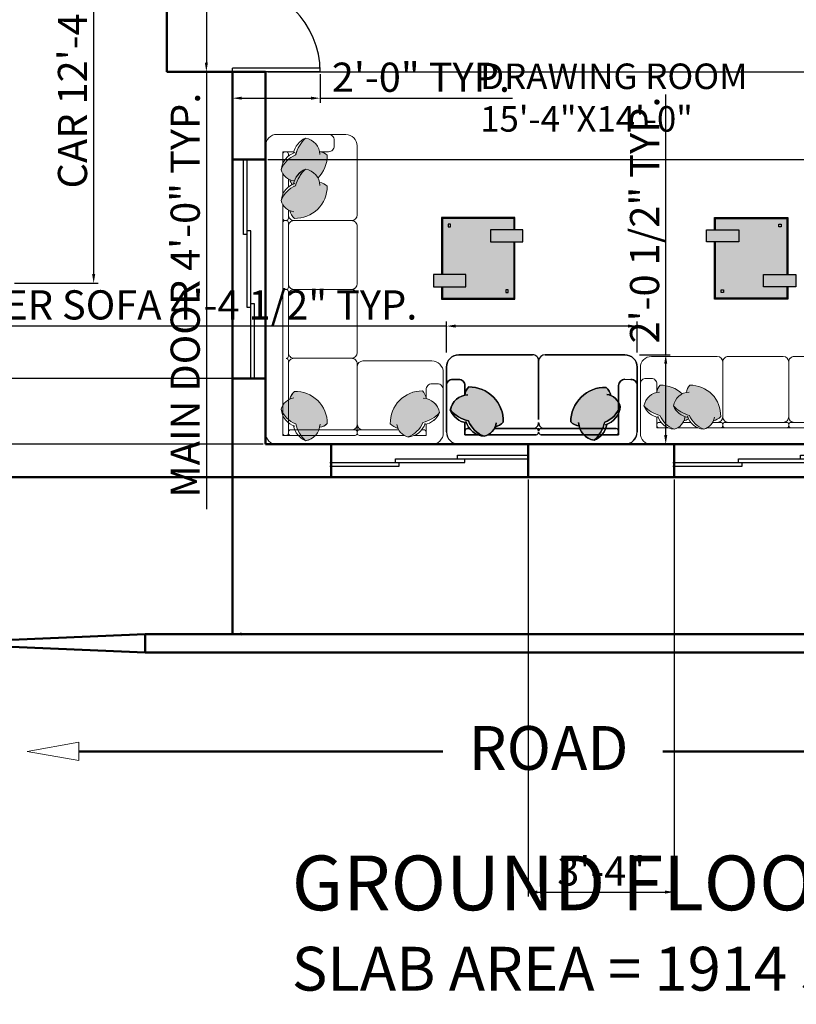
# Model space of a CAD drawing. Units: inches. Extents: x 1913 to 5309, y 1003 to 1733.
# Tile 2 of 23: x 2090 to 2303, y 1003 to 1272. Entities that reach past the tile are written whole.
import ezdxf

# ---------------------------------------------------------------- set-up
doc = ezdxf.new("R2010")
doc.units = ezdxf.units.IN
for name, color, linetype, lineweight in [('A-ANNO-DIMS', 2, 'Continuous', 18), ('A-ANNO-SYMB', 1, 'Continuous', 18), ('A-ANNO-TEXT', 7, 'Continuous', 18), ('A-AREA-IDEN', 3, 'Continuous', 18), ('A-DOOR', 4, 'Continuous', 25), ('A-FURN', 8, 'Continuous', 18), ('A-GLAZ', 5, 'Continuous', 25), ('A-WALL', 7, 'Continuous', 50)]:
    doc.layers.add(name, color=color, linetype=linetype, lineweight=lineweight)
doc.layers.add('MOBIL', color=7, linetype='Continuous')
doc.styles.get("Standard").update_dxf_attribs({"font": 'arial.ttf'})
doc.dimstyles.new('ISO-25', dxfattribs={"dimtxt": 8, "dimasz": 2.5, "dimexe": 1.25, "dimexo": 0.625, "dimtad": 1, "dimdec": 1, "dimlunit": 3, "dimtxsty": 'Standard', "dimcen": 2.5, "dimclrd": 256, "dimclrt": 1, "dimadec": 0, "dimazin": 0, "dimtfac": 1, "dimtdec": 1, "dimtmove": 0, "dimatfit": 3, "dimfxl": 1, "dimarcsym": 0})

# ---------------------------------------------------------------- blocks, each defined once
blk = doc.blocks.new("MD D 4'")
for p, q in [((0, 24), (0, 0)), ((1, 24), (1, 0)), ((47, 24), (47, 0)), ((48, 24), (48, 0)), ((0, 0), (1, 0)), ((48, 0), (47, 0))]:
    blk.add_line(p, q)
for centre, start, end in [((0, 0), 0, 90), ((48, 0), 90, 180)]:
    blk.add_arc(centre, 24, start, end)
blk = doc.blocks.new('Mesa de centro Cantria feeling')
at = {"layer": 'MOBIL', "ltscale": 0.2}
h = blk.add_hatch(color=256, dxfattribs=at)
h.set_gradient(color1=(74, 55, 38), color2=(104, 77, 54), one_color=1, tint=0.31, name='CYLINDER')
h.paths.add_polyline_path([(-0.85, -0.3), (-0.7, -0.3), (-0.7, 0.1), (-0.85, 0.1)])
h = blk.add_hatch(color=256, dxfattribs=at)
h.set_gradient(color1=(221, 221, 223), one_color=1, tint=1)
h.paths.add_polyline_path([(-0.15, -0.6), (-0.15, -0.89), (-0.01, -0.89), (-0.01, -0.01), (-0.7, -0.01), (-0.7, -0.3), (-0.85, -0.3), (-0.85, -0.01), (-0.99, -0.01), (-0.99, -0.89), (-0.3, -0.89), (-0.3, -0.6)])
h.paths.add_polyline_path([(-0.112, -0.112), (-0.112, -0.082), (-0.082, -0.082), (-0.082, -0.112)], flags=16)
h.paths.add_polyline_path([(-0.888, -0.788), (-0.888, -0.818), (-0.918, -0.818), (-0.918, -0.788)], flags=16)
h = blk.add_hatch(color=256, dxfattribs=at)
h.set_gradient(color1=(74, 55, 38), color2=(104, 77, 54), one_color=1, tint=0.31, name='CYLINDER')
h.paths.add_polyline_path([(-0.15, -0.6), (-0.3, -0.6), (-0.3, -1), (-0.15, -1)])
for points in [[(-0.85, 0), (-1, 0), (-1, -0.9), (-0.3, -0.9)], [(-0.15, -0.9), (0, -0.9), (0, 0), (-0.7, 0)], [(-0.85, -0.01), (-0.99, -0.01), (-0.99, -0.89), (-0.3, -0.89)], [(-0.15, -0.89), (-0.01, -0.89), (-0.01, -0.01), (-0.7, -0.01)]]:
    blk.add_lwpolyline(points, dxfattribs=at)
for points in [[(-0.85, -0.3), (-0.7, -0.3), (-0.7, 0.1), (-0.85, 0.1)], [(-0.082, -0.082), (-0.112, -0.082), (-0.112, -0.112), (-0.082, -0.112)], [(-0.15, -0.6), (-0.3, -0.6), (-0.3, -1), (-0.15, -1)], [(-0.918, -0.818), (-0.888, -0.818), (-0.888, -0.788), (-0.918, -0.788)]]:
    blk.add_lwpolyline(points, close=True, dxfattribs=at)
blk = doc.blocks.new('d2 s')
at = {"transparency": 33554687}
h = blk.add_hatch(color=256, dxfattribs=at)
h.dxf.hatch_style = 1
h.paths.add_polyline_path([(3953.01, 1202.6, 0.213835), (3948.73, 1198.21, 0.233217), (3951.28, 1195.23, 0.122039), (3952.62, 1192.95, 0.425972), (3962.37, 1202.51, 0.156703), (3960.25, 1203.55), (3960.12, 1203.55, 0.310469), (3955.94, 1207.57, 0.147724)])
h = blk.add_hatch(color=256, dxfattribs=at)
h.dxf.hatch_style = 1
h.paths.add_polyline_path([(3953.9, 1162.75, -0.084911), (3952.59, 1164.92, -0.046133), (3950.85, 1165.51), (3950.85, 1171.8, -0.039409), (3951.63, 1172.02, -0.165523), (3952.68, 1174.28, -0.42585), (3962.24, 1164.53, -0.121928), (3959.96, 1163.19, -0.027403), (3959.75, 1162.75)])
h.paths.add_polyline_path([(3949.17, 1166.48), (3949.17, 1170.75, -0.097704), (3950.85, 1171.8), (3950.85, 1165.51, -0.04873)])
h.paths.add_polyline_path([(3947.62, 1167.84, -0.16488), (3949.17, 1170.75), (3949.17, 1166.48, -0.051917)])
h.paths.add_polyline_path([(3956, 1161.07, -0.090388), (3953.9, 1162.75), (3959.75, 1162.75, -0.136035), (3958.07, 1161.07)])
blk.add_line((3946.53, 1205.25), (3946.53, 1159.36), dxfattribs=at)
for p, q in [((3949.84, 1161.07), (3950.18, 1161.07)), ((3964.47, 1159.37), (3964.46, 1157.65))]:
    blk.add_line(p, q)
for points in [[(3949.93, 1208.66), (3967.86, 1208.66)], [(3964.46, 1205.25), (3964.46, 1206.96)], [(3971.27, 1205.25), (3971.27, 1184.84)], [(3949.17, 1203.55), (3952.49, 1203.55), (3949.17, 1203.55), (3949.17, 1199.96)], [(3950.85, 1202.87), (3950.85, 1202.25)], [(3960.13, 1203.55), (3962.77, 1203.55)], [(3949.17, 1197.14), (3949.17, 1183.83)], [(3950.85, 1195.43), (3950.85, 1183.83)], [(3949.17, 1164.09), (3949.17, 1182.51)], [(3950.99, 1183.17), (3950.65, 1183.17)], [(3950.85, 1161.74), (3950.85, 1182.51)], [(3969.63, 1183.17), (3953.36, 1183.17)], [(3971.25, 1181.39), (3971.25, 1159.35)], [(3949.17, 1161.07), (3949.17, 1164.4), (3949.17, 1161.07), (3952.75, 1161.07)], [(3952.75, 1161.06), (3962.77, 1161.06)], [(3949.93, 1155.95), (3967.86, 1155.95)]]:
    blk.add_lwpolyline(points, close=True, dxfattribs=at)
for points in [[(3962.76, 1208.66, -0.414214), (3964.46, 1206.97, 0.414214)], [(3967.85, 1208.66, -0.414212), (3971.25, 1205.26, 0.414212)], [(3964.46, 1205.26, -0.414214), (3962.76, 1203.57, 0.414214)], [(3950.18, 1203.55, -0.414214), (3950.85, 1202.88, 0.414214)], [(3964.47, 1159.37, 0.414214), (3962.77, 1161.06, -0.414214)], [(3967.85, 1155.95, 0.414212), (3971.25, 1159.35, -0.414212)], [(3962.76, 1155.95, 0.414214), (3964.46, 1157.65, -0.414214)]]:
    blk.add_lwpolyline(points, format="xyb", close=True, dxfattribs=at)
for points in [[(3955.94, 1207.57, 0.147724), (3953.01, 1202.6, 0.213355), (3948.73, 1198.22, -0.213355), (3953.01, 1202.6, -0.147724), (3955.94, 1207.57, 0.249545), (3952.4, 1203.17, -0.249545), (3955.93, 1207.59, -0.356779), (3960.22, 1202.7, 0.356779), (3955.94, 1207.57)], [(3948.72, 1198.23, 0.306333), (3952.42, 1194.91, -0.306333), (3948.72, 1198.23, -0.306674), (3952.79, 1203.29, 0.306674), (3948.72, 1198.23)], [(3952.62, 1192.95, 0.425972), (3962.37, 1202.51, 0.165552), (3960.12, 1203.57, -0.165552), (3962.37, 1202.51, -0.425972), (3952.63, 1192.95, -0.121514), (3951.29, 1195.22, 0.121514), (3952.62, 1192.95)], [(3962.24, 1164.53, 0.425972), (3952.68, 1174.28, 0.165552), (3951.63, 1172.02, -0.165552), (3952.68, 1174.28, -0.425972), (3962.24, 1164.53, -0.121514), (3959.97, 1163.19, 0.121514), (3962.24, 1164.53)], [(3947.62, 1167.84, 0.147724), (3952.59, 1164.92, 0.213355), (3956.97, 1160.64, -0.213355), (3952.59, 1164.92, -0.147724), (3947.62, 1167.84, 0.249545), (3952.02, 1164.3, -0.249545), (3947.61, 1167.84, -0.356779), (3952.49, 1172.13, 0.356779), (3947.62, 1167.84)], [(3956.96, 1160.63, 0.306333), (3960.28, 1164.33, -0.306333), (3956.96, 1160.63, -0.306674), (3951.9, 1164.7, 0.306674), (3956.96, 1160.63)]]:
    blk.add_lwpolyline(points, format="xyb", dxfattribs=at)
for centre, radius, start, end in [((3949.93, 1205.26), 3.4, 90.0002, 179.9998), ((3949.93, 1205.26), 3.4, 90.0846, 180.0842), ((3949.85, 1183.85), 0.681, 179.1575, 269.1575), ((3950.18, 1183.84), 0.671, 270, 0), ((3950.18, 1183.84), 0.671, 270, 0), ((3952.51, 1184.83), 1.66, 179.4889, 271.234), ((3969.59, 1184.83), 1.66, 268.766, 0.5111), ((3969.59, 1184.83), 1.66, 268.7816, 0.5111), ((3949.85, 1182.49), 0.681, 90.8425, 180.8425), ((3950.18, 1182.5), 0.671, 360, 90), ((3950.18, 1182.5), 0.671, 360, 90), ((3952.51, 1181.52), 1.66, 88.766, 180.5111), ((3969.39, 1181.32), 1.86, 2.0577, 84.9818), ((3969.39, 1181.32), 1.86, 2.0577, 84.9818), ((3949.84, 1161.74), 0.671, 180, 270), ((3950.18, 1161.74), 0.671, 270, 0), ((3949.93, 1159.36), 3.4, 180.0002, 269.9998), ((3949.93, 1159.37), 3.4, 180.0846, 270.0842)]:
    blk.add_arc(centre, radius, start, end, dxfattribs=at)
blk = doc.blocks.new('SOFA 1')
at = {"transparency": 33554687}
h = blk.add_hatch(color=256, dxfattribs=at)
h.dxf.hatch_style = 1
h.paths.add_polyline_path([(3769.65, 1307.6, 0.084911), (3767.15, 1309.12, 0.046133), (3766.46, 1311.13), (3759.18, 1311.13, 0.039409), (3758.92, 1310.24, 0.165523), (3756.31, 1309.02, 0.42585), (3767.59, 1297.95, 0.121928), (3769.15, 1300.58, 0.027403), (3769.65, 1300.83)])
h.paths.add_polyline_path([(3765.34, 1313.08), (3760.4, 1313.08, 0.097704), (3759.18, 1311.13), (3766.46, 1311.13, 0.04873)])
h.paths.add_polyline_path([(3763.76, 1314.88, 0.16488), (3760.4, 1313.08), (3765.34, 1313.08, 0.051917)])
h.paths.add_polyline_path([(3771.6, 1305.17, 0.090388), (3769.65, 1307.6), (3769.65, 1300.83, 0.136035), (3771.6, 1302.77)])
h = blk.add_hatch(color=256, dxfattribs=at)
h.dxf.hatch_style = 1
h.paths.add_polyline_path([(3723.52, 1308.63, 0.147724), (3717.76, 1305.24, 0.310469), (3722.42, 1300.4), (3722.42, 1300.25, 0.156703), (3723.62, 1297.8, 0.425821), (3734.69, 1309.08, 0.121928), (3732.05, 1310.63, 0.233216), (3728.6, 1313.59, 0.213835)])
h = blk.add_hatch(color=256, dxfattribs=at)
h.dxf.hatch_style = 1
h.paths.add_polyline_path([(3769.16, 1235.96, 0.122267), (3767.6, 1238.61, 0.425972), (3756.32, 1227.54, 0.165563), (3758.93, 1226.32, 0.309481), (3763.76, 1221.69, 0.002677), (3763.83, 1221.72, 0.146094), (3767.16, 1227.43, 0.212433), (3772.1, 1232.48, 0.235342)])
h = blk.add_hatch(color=256, dxfattribs=at)
h.dxf.hatch_style = 1
h.paths.add_polyline_path([(3769.16, 1225.36, 0.122267), (3767.6, 1228.01, 0.425972), (3756.32, 1216.94, 0.165563), (3758.93, 1215.72, 0.309481), (3763.76, 1211.09, 0.002677), (3763.83, 1211.12, 0.146094), (3767.16, 1216.83, 0.212433), (3772.1, 1221.88, 0.235342)])
for p, q in [((3720.45, 1316.13), (3773.58, 1316.13)), ((3777.51, 1312.19), (3777.51, 1213.72))]:
    blk.add_line(p, q, dxfattribs=at)
for points in [[(3763.76, 1314.88, -0.147724), (3767.15, 1309.12, -0.213355), (3772.1, 1304.05, 0.213355), (3767.15, 1309.12, 0.147724), (3763.76, 1314.88, -0.249545), (3767.86, 1309.77, 0.249545), (3763.77, 1314.89, 0.356779), (3758.8, 1309.23, -0.356779), (3763.76, 1314.88)], [(3717.76, 1305.24, -0.147724), (3723.52, 1308.63, -0.213355), (3728.59, 1313.59, 0.213355), (3723.52, 1308.63, 0.147724), (3717.76, 1305.24, -0.249545), (3722.86, 1309.34, 0.249545), (3717.75, 1305.25, 0.356779), (3723.4, 1300.28, -0.356779), (3717.76, 1305.24)], [(3734.69, 1309.08, -0.425972), (3723.62, 1297.8, -0.165552), (3722.4, 1300.4, 0.165552), (3723.62, 1297.79, 0.425972), (3734.69, 1309.07, 0.121514), (3732.07, 1310.63, -0.121514), (3734.69, 1309.08)], [(3728.58, 1313.6, -0.306333), (3732.42, 1309.31, 0.306333), (3728.58, 1313.6, 0.306674), (3722.72, 1308.89, -0.306674), (3728.58, 1313.6)], [(3767.6, 1297.95, -0.425972), (3756.31, 1309.01, -0.165552), (3758.92, 1310.24, 0.165552), (3756.31, 1309.02, 0.425972), (3767.59, 1297.95, 0.121514), (3769.14, 1300.57, -0.121514), (3767.6, 1297.95)], [(3772.11, 1304.06, -0.306333), (3767.83, 1300.22, 0.306333), (3772.11, 1304.06, 0.306674), (3767.4, 1309.91, -0.306674), (3772.11, 1304.06)], [(3770.44, 1286.63, -0.414214), (3769.66, 1287.4, 0.414214), (3770.44, 1286.63, 0.414214), (3769.66, 1285.83, -0.414214), (3770.44, 1286.63)], [(3748.01, 1262.99, -0.414214), (3746.05, 1264.95, 0.414214), (3748.01, 1262.97, 0.414213), (3746.05, 1261.01, -0.414213), (3748.01, 1262.99)], [(3770.44, 1262.99, -0.414214), (3769.66, 1263.77, 0.414214), (3770.44, 1262.99, 0.414214), (3769.66, 1262.19, -0.414214), (3770.44, 1262.99)], [(3770.83, 1262.97, -0.414214), (3771.61, 1262.19, 0.414214), (3770.83, 1262.99, 0.414214), (3771.61, 1263.77, -0.414214), (3770.83, 1262.97)], [(3748.01, 1239.35, -0.414214), (3746.05, 1241.31, 0.414214), (3748.01, 1239.33, 0.414213), (3746.05, 1237.37, -0.414213), (3748.01, 1239.35)], [(3767.7, 1239.33, -0.414214), (3769.66, 1237.37, 0.414214), (3767.7, 1239.35, 0.414214), (3769.66, 1241.31, -0.414214), (3767.7, 1239.33)], [(3770.44, 1239.35, -0.414214), (3769.66, 1240.13, 0.414214), (3770.44, 1239.33, 0.414214), (3769.66, 1238.55, -0.414214), (3770.44, 1239.35)], [(3770.83, 1239.33, -0.414214), (3771.61, 1238.55, 0.414214), (3770.83, 1239.35, 0.414214), (3771.61, 1240.13, -0.414214), (3770.83, 1239.33)], [(3756.32, 1227.54, -0.425972), (3767.6, 1238.61, -0.121514), (3769.16, 1235.98, 0.121514), (3767.6, 1238.61, 0.425972), (3756.32, 1227.54, 0.165552), (3758.93, 1226.32, -0.165552), (3756.32, 1227.54)], [(3772.1, 1232.5, -0.306674), (3767.41, 1226.64, 0.306674), (3772.1, 1232.5, 0.306333), (3767.84, 1236.34, -0.306333), (3772.1, 1232.5)], [(3763.78, 1221.67, 0.249545), (3767.87, 1226.78, -0.249545), (3763.76, 1221.69, -0.356779), (3758.81, 1227.32, 0.356779), (3763.77, 1221.68, 0.147724), (3767.16, 1227.43, 0.213355), (3772.11, 1232.51, -0.213355), (3767.16, 1227.43, -0.147724), (3763.78, 1221.67)], [(3756.32, 1216.94, -0.200233), (3759.49, 1224.76, 0.200233), (3756.32, 1216.94, 0.165552), (3758.93, 1215.72, -0.165552), (3756.32, 1216.94)], [(3772.1, 1221.9, -0.306674), (3767.41, 1216.04, 0.306674), (3772.1, 1221.9, -0.213355), (3767.16, 1216.83, -0.147724), (3763.77, 1211.08, 0.147724), (3767.15, 1216.83, 0.213355), (3772.1, 1221.9)], [(3763.76, 1211.09, -0.356779), (3758.81, 1216.72, 0.356779), (3763.76, 1211.09, 0.249545), (3767.87, 1216.18, -0.249545), (3763.76, 1211.09)]]:
    blk.add_lwpolyline(points, format="xyb", dxfattribs=at)
for points in [[(3716.51, 1312.2), (3716.51, 1291.44)], [(3722.42, 1313.08), (3722.42, 1309.23), (3722.42, 1313.08), (3726.57, 1313.08)], [(3723.21, 1311.13), (3723.93, 1311.13)], [(3729.85, 1313.08), (3745.25, 1313.08)], [(3731.82, 1311.13), (3745.25, 1311.13)], [(3746.01, 1312.3), (3746.01, 1288.55)], [(3746.01, 1310.97), (3746.01, 1311.36)], [(3768.11, 1313.08), (3746.78, 1313.08)], [(3768.87, 1311.13), (3746.78, 1311.13)], [(3771.6, 1313.08), (3767.75, 1313.08), (3771.6, 1313.08), (3771.6, 1308.93)], [(3769.66, 1287.39), (3769.65, 1312.3)], [(3771.6, 1313.08), (3771.61, 1233.74)], [(3746.01, 1288.54), (3746.01, 1308.23)], [(3769.65, 1309.43), (3769.65, 1308.71)], [(3722.42, 1300.39), (3722.42, 1297.33)], [(3720.45, 1295.38), (3718.48, 1295.38)], [(3720.45, 1287.5), (3744.09, 1287.5)], [(3746.02, 1284.63), (3746.02, 1264.94)], [(3747.99, 1286.6), (3767.69, 1286.6)], [(3769.66, 1263.75), (3769.66, 1285.81)], [(3769.66, 1277.18), (3769.66, 1263.75)], [(3746.02, 1260.99), (3746.02, 1241.3)], [(3747.99, 1262.97), (3767.69, 1262.97)], [(3769.66, 1240.12), (3769.66, 1262.18)], [(3770.43, 1262.97), (3770.82, 1262.97)], [(3746.02, 1237.36), (3746.02, 1213.74)], [(3747.99, 1239.33), (3767.69, 1239.33)], [(3769.66, 1235.71), (3769.66, 1238.54)], [(3770.43, 1239.33), (3770.82, 1239.33)], [(3771.61, 1223.14), (3771.61, 1230.47)], [(3769.66, 1225.11), (3769.66, 1227.82)], [(3767.76, 1215.72), (3771.61, 1215.72), (3771.61, 1219.84), (3771.61, 1215.72)], [(3769.66, 1216.5), (3769.66, 1217.22)], [(3753.91, 1211.77), (3753.91, 1213.74)], [(3755.86, 1215.72), (3758.92, 1215.72)], [(3749.97, 1209.8), (3773.58, 1209.8)]]:
    blk.add_lwpolyline(points, close=True, dxfattribs=at)
for points in [[(3722.42, 1311.91, 0.414214), (3723.2, 1311.13, -0.414214)], [(3770.43, 1313.08, 0.414214), (3769.65, 1312.3, -0.414214)], [(3771.6, 1312.3, 0.414214), (3770.82, 1313.08, -0.414214)], [(3716.51, 1297.34, 0.414214), (3718.47, 1295.38, -0.414214)], [(3720.44, 1295.38, 0.414214), (3722.4, 1297.34, -0.414214)], [(3716.51, 1291.45, 0.414212), (3720.44, 1287.52, -0.414212)], [(3746.03, 1288.56, 0.414214), (3747.99, 1286.6, 0.414213), (3746.03, 1284.64, -0.414213), (3747.99, 1286.6, -0.414214)], [(3769.66, 1284.64, 0.414214), (3767.7, 1286.6, 0.414214), (3769.66, 1288.56, -0.414214), (3767.7, 1286.6, -0.414214)], [(3769.66, 1261.01, 0.414214), (3767.7, 1262.97, 0.414214), (3769.66, 1264.93, -0.414214), (3767.7, 1262.97, -0.414214)], [(3769.16, 1225.36, 0.071861), (3768.39, 1227.01, -0.071861)], [(3772.13, 1221.9, 0.306333), (3767.84, 1225.74, -0.306333)], [(3769.66, 1216.52, 0.414214), (3770.44, 1215.74, -0.414214)], [(3770.83, 1215.74, 0.414214), (3771.61, 1216.52, -0.414214)], [(3746.05, 1213.76, 0.414212), (3749.98, 1209.82, -0.414212)], [(3755.87, 1215.72, 0.414214), (3753.91, 1213.76, -0.414214)], [(3755.87, 1209.8, -0.414214), (3753.91, 1211.76, 0.414214)]]:
    blk.add_lwpolyline(points, format="xyb", close=True, dxfattribs=at)
for centre, radius, start, end in [((3720.44, 1312.2), 3.93, 90.0002, 179.9998), ((3720.44, 1312.19), 3.94, 89.9158, 179.9154), ((3773.58, 1312.2), 3.93, 0.0002, 89.9998), ((3773.57, 1312.19), 3.94, 359.9158, 89.9154), ((3744.09, 1309.21), 1.92, 358.766, 90.5111), ((3745.22, 1312.29), 0.789, 0.8425, 90.8425), ((3745.24, 1311.91), 0.777, 270, 0), ((3745.24, 1311.91), 0.777, 270, 0), ((3746.8, 1312.29), 0.789, 89.1575, 179.1575), ((3746.79, 1311.91), 0.777, 180, 270), ((3746.79, 1311.91), 0.777, 180, 270), ((3747.93, 1309.21), 1.92, 89.4889, 181.234), ((3768.87, 1312.3), 0.777, 360, 90), ((3768.87, 1311.91), 0.777, 270, 0), ((3744.08, 1289.48), 1.96, 270, 360), ((3744.08, 1289.48), 1.96, 270, 360), ((3773.58, 1213.73), 3.93, 270.0002, 359.9998), ((3773.59, 1213.73), 3.93, 269.9156, 359.9152)]:
    blk.add_arc(centre, radius, start, end, dxfattribs=at)
blk = doc.blocks.new('*D21')
at = {"layer": 'A-ANNO-DIMS', "color": 0, "lineweight": -2, "transparency": 16777216}
for p, q in [((2148.37, 1104.59), (2148.37, 1105.21)), ((2503.87, 1103.96), (2150.87, 1103.96)), ((2506.37, 1104.59), (2506.37, 1105.21))]:
    blk.add_line(p, q, dxfattribs=at)
at = {"layer": 'A-ANNO-DIMS', "color": 0, "transparency": 16777216}
for points in [[(2150.87, 1104.38), (2150.87, 1103.55), (2148.37, 1103.96)], [(2503.87, 1104.38), (2503.87, 1103.55), (2506.37, 1103.96)]]:
    blk.add_solid(points, dxfattribs=at)
at = {"layer": 'Defpoints', "color": 0, "transparency": 16777216}
for p in [(2148.37, 1103.96), (2148.37, 1103.96), (2506.37, 1103.96)]:
    blk.add_point(p, dxfattribs=at)
at = {"layer": 'A-ANNO-DIMS', "color": 0, "transparency": 16777216, "insert": (2327.37, 1108.67), "char_height": 8, "attachment_point": 5}
blk.add_mtext('29\'-10"', dxfattribs=at)
blk = doc.blocks.new('WIN-54')
for p, q in [((0, 54), (0, 35)), ((1, 54), (1, 17)), ((1, 36), (2, 36)), ((2, 36), (2, 0)), ((0, 35), (1, 35)), ((2, 19), (3, 19)), ((3, 19), (3, 0)), ((1, 17), (2, 17))]:
    blk.add_line(p, q)
blk = doc.blocks.new('WIN-60')
for p, q in [((0, 60), (0, 39.5)), ((1, 60), (1, 19.5)), ((1, 40.5), (2, 40.5)), ((2, 40.5), (2, 0)), ((0, 39.5), (1, 39.5)), ((1, 19.5), (2, 19.5)), ((2, 20.5), (3, 20.5)), ((3, 20.5), (3, 0))]:
    blk.add_line(p, q)
blk = doc.blocks.new('*D77')
at = {"layer": 'A-ANNO-DIMS', "color": 0, "lineweight": -2, "transparency": 16777216}
for p, q in [((2206.96, 1181.12), (2206.96, 1189.59)), ((2259.21, 1181.12), (2259.21, 1189.59))]:
    blk.add_line(p, q, dxfattribs=at)
at = {"layer": 'A-ANNO-DIMS', "lineweight": -2, "transparency": 16777216}
for p, q in [((2206.96, 1188.34), (2044.37, 1188.34)), ((2256.71, 1188.34), (2209.46, 1188.34))]:
    blk.add_line(p, q, dxfattribs=at)
at = {"layer": 'A-ANNO-DIMS', "transparency": 16777216}
for points in [[(2209.46, 1188.75), (2209.46, 1187.92), (2206.96, 1188.34)], [(2256.71, 1188.75), (2256.71, 1187.92), (2259.21, 1188.34)]]:
    blk.add_solid(points, dxfattribs=at)
at = {"layer": 'Defpoints', "color": 0, "transparency": 16777216}
for p in [(2206.96, 1188.34), (2206.96, 1180.5), (2259.21, 1180.5)]:
    blk.add_point(p, dxfattribs=at)
at = {"layer": 'A-ANNO-DIMS', "color": 1, "transparency": 16777216, "insert": (2124.42, 1193.1), "char_height": 8, "attachment_point": 5}
blk.add_mtext('2-SEATER SOFA 4\'-4 1/2" TYP.', dxfattribs=at)
blk = doc.blocks.new('*D78')
at = {"layer": 'A-ANNO-DIMS', "lineweight": -2, "transparency": 16777216}
for p, q in [((2267.05, 1180.5), (2267.05, 1251.79)), ((2267.05, 1158.47), (2267.05, 1178))]:
    blk.add_line(p, q, dxfattribs=at)
at = {"layer": 'A-ANNO-DIMS', "color": 0, "lineweight": -2, "transparency": 16777216}
for p, q in [((2259.84, 1180.5), (2268.3, 1180.5)), ((2259.84, 1155.97), (2268.3, 1155.97))]:
    blk.add_line(p, q, dxfattribs=at)
at = {"layer": 'A-ANNO-DIMS', "transparency": 16777216}
for points in [[(2266.63, 1178), (2267.47, 1178), (2267.05, 1180.5)], [(2266.63, 1158.47), (2267.47, 1158.47), (2267.05, 1155.97)]]:
    blk.add_solid(points, dxfattribs=at)
at = {"layer": 'Defpoints', "color": 0, "transparency": 16777216}
for p in [(2259.21, 1180.5), (2267.05, 1180.5), (2259.21, 1155.97)]:
    blk.add_point(p, dxfattribs=at)
at = {"layer": 'A-ANNO-DIMS', "color": 1, "transparency": 16777216, "insert": (2262.29, 1217.39), "char_height": 8, "attachment_point": 5, "rotation": 90}
blk.add_mtext('2\'-0 1/2" TYP.', dxfattribs=at)
blk = doc.blocks.new('*D81')
at = {"layer": 'A-ANNO-DIMS', "color": 0, "lineweight": -2, "transparency": 16777216}
for p, q in [((2147.75, 1305.96), (2139.92, 1305.96)), ((2147.75, 1257.96), (2139.92, 1257.96))]:
    blk.add_line(p, q, dxfattribs=at)
at = {"layer": 'A-ANNO-DIMS', "lineweight": -2, "transparency": 16777216}
for p, q in [((2141.17, 1303.46), (2141.17, 1260.46)), ((2141.17, 1257.96), (2141.17, 1138.14))]:
    blk.add_line(p, q, dxfattribs=at)
at = {"layer": 'A-ANNO-DIMS', "transparency": 16777216}
for points in [[(2140.76, 1303.46), (2141.59, 1303.46), (2141.17, 1305.96)], [(2140.76, 1260.46), (2141.59, 1260.46), (2141.17, 1257.96)]]:
    blk.add_solid(points, dxfattribs=at)
at = {"layer": 'Defpoints', "color": 0, "transparency": 16777216}
for p in [(2148.37, 1305.96), (2141.17, 1257.96), (2148.37, 1257.96)]:
    blk.add_point(p, dxfattribs=at)
at = {"layer": 'A-ANNO-DIMS', "color": 1, "transparency": 16777216, "insert": (2136.41, 1196.8), "char_height": 8, "attachment_point": 5, "rotation": 90}
blk.add_mtext('MAIN DOOR 4\'-0" TYP.', dxfattribs=at)
blk = doc.blocks.new('*D82')
at = {"layer": 'A-ANNO-DIMS', "color": 0, "lineweight": -2, "transparency": 16777216}
for p, q in [((2148.37, 1257.34), (2148.37, 1249.51)), ((2172.37, 1257.34), (2172.37, 1249.51))]:
    blk.add_line(p, q, dxfattribs=at)
at = {"layer": 'A-ANNO-DIMS', "lineweight": -2, "transparency": 16777216}
for p, q in [((2150.87, 1250.76), (2169.87, 1250.76)), ((2172.37, 1250.76), (2225.02, 1250.76))]:
    blk.add_line(p, q, dxfattribs=at)
at = {"layer": 'A-ANNO-DIMS', "transparency": 16777216}
for points in [[(2150.87, 1251.18), (2150.87, 1250.35), (2148.37, 1250.76)], [(2169.87, 1251.18), (2169.87, 1250.35), (2172.37, 1250.76)]]:
    blk.add_solid(points, dxfattribs=at)
at = {"layer": 'Defpoints', "color": 0, "transparency": 16777216}
for p in [(2148.37, 1257.96), (2172.37, 1257.96), (2172.37, 1250.76)]:
    blk.add_point(p, dxfattribs=at)
at = {"layer": 'A-ANNO-DIMS', "color": 1, "transparency": 16777216, "insert": (2199.95, 1255.47), "char_height": 8, "attachment_point": 5}
blk.add_mtext('2\'-0" TYP.', dxfattribs=at)
blk = doc.blocks.new('*D85')
at = {"layer": 'A-ANNO-DIMS', "color": 0, "lineweight": -2, "transparency": 16777216}
for p, q in [((2088.63, 1348.67), (2111.54, 1348.67)), ((2088.63, 1200.09), (2111.54, 1200.09))]:
    blk.add_line(p, q, dxfattribs=at)
at = {"layer": 'A-ANNO-DIMS', "lineweight": -2, "transparency": 16777216}
blk.add_line((2110.29, 1346.17), (2110.29, 1202.59), dxfattribs=at)
at = {"layer": 'A-ANNO-DIMS', "transparency": 16777216}
for points in [[(2109.87, 1346.17), (2110.71, 1346.17), (2110.29, 1348.67)], [(2109.87, 1202.59), (2110.71, 1202.59), (2110.29, 1200.09)]]:
    blk.add_solid(points, dxfattribs=at)
at = {"layer": 'Defpoints', "color": 0, "transparency": 16777216}
for p in [(2088, 1348.67), (2088, 1200.09), (2110.29, 1200.09)]:
    blk.add_point(p, dxfattribs=at)
at = {"layer": 'A-ANNO-DIMS', "color": 1, "transparency": 16777216, "insert": (2105.53, 1274.38), "char_height": 8, "attachment_point": 5, "rotation": 90}
blk.add_mtext('CAR 12\'-4 1/2" TYP.', dxfattribs=at)
blk = doc.blocks.new('*D98')
at = {"layer": 'A-ANNO-DIMS', "color": 0, "lineweight": -2, "transparency": 16777216}
for p, q in [((2229.37, 1146.34), (2229.37, 1032.04)), ((2269.37, 1146.34), (2269.37, 1032.04))]:
    blk.add_line(p, q, dxfattribs=at)
at = {"layer": 'A-ANNO-DIMS', "lineweight": -2, "transparency": 16777216}
blk.add_line((2231.87, 1033.29), (2266.87, 1033.29), dxfattribs=at)
at = {"layer": 'A-ANNO-DIMS', "transparency": 16777216}
for points in [[(2231.87, 1033.7), (2231.87, 1032.87), (2229.37, 1033.29)], [(2266.87, 1033.7), (2266.87, 1032.87), (2269.37, 1033.29)]]:
    blk.add_solid(points, dxfattribs=at)
at = {"layer": 'Defpoints', "color": 0, "transparency": 16777216}
for p in [(2229.37, 1146.96), (2269.37, 1146.96), (2269.37, 1033.29)]:
    blk.add_point(p, dxfattribs=at)
at = {"layer": 'A-ANNO-DIMS', "color": 1, "transparency": 16777216, "insert": (2249.37, 1038), "char_height": 8, "attachment_point": 5}
blk.add_mtext('3\'-4"', dxfattribs=at)
blk = doc.blocks.new('*D100')
at = {"layer": 'A-ANNO-DIMS', "lineweight": -2, "transparency": 16777216}
for p, q in [((1923.37, 1173.96), (1923.37, 1198.23)), ((1923.37, 1158.46), (1923.37, 1171.46))]:
    blk.add_line(p, q, dxfattribs=at)
at = {"layer": 'A-ANNO-DIMS', "color": 0, "lineweight": -2, "transparency": 16777216}
for p, q in [((2156.75, 1173.96), (1922.12, 1173.96)), ((2156.75, 1155.96), (1922.12, 1155.96))]:
    blk.add_line(p, q, dxfattribs=at)
at = {"layer": 'A-ANNO-DIMS', "transparency": 16777216}
for points in [[(1922.96, 1171.46), (1923.79, 1171.46), (1923.37, 1173.96)], [(1922.96, 1158.46), (1923.79, 1158.46), (1923.37, 1155.96)]]:
    blk.add_solid(points, dxfattribs=at)
at = {"layer": 'Defpoints', "color": 0, "transparency": 16777216}
for p in [(1923.37, 1173.96), (2157.37, 1173.96), (2157.37, 1155.96)]:
    blk.add_point(p, dxfattribs=at)
at = {"layer": 'A-ANNO-DIMS', "color": 1, "transparency": 16777216, "insert": (1918.66, 1187.35), "char_height": 8, "attachment_point": 5, "rotation": 90}
blk.add_mtext('1\'-6"', dxfattribs=at)
blk = doc.blocks.new('*D101')
at = {"layer": 'A-ANNO-DIMS', "color": 0, "lineweight": -2, "transparency": 16777216}
for p, q in [((2158, 1257.96), (2548.62, 1257.96)), ((2158, 1233.96), (2548.62, 1233.96))]:
    blk.add_line(p, q, dxfattribs=at)
at = {"layer": 'A-ANNO-DIMS', "lineweight": -2, "transparency": 16777216}
blk.add_line((2547.37, 1255.46), (2547.37, 1236.46), dxfattribs=at)
at = {"layer": 'A-ANNO-DIMS', "transparency": 16777216}
for points in [[(2546.96, 1255.46), (2547.79, 1255.46), (2547.37, 1257.96)], [(2546.96, 1236.46), (2547.79, 1236.46), (2547.37, 1233.96)]]:
    blk.add_solid(points, dxfattribs=at)
at = {"layer": 'Defpoints', "color": 0, "transparency": 16777216}
for p in [(2157.37, 1257.96), (2157.37, 1233.96), (2547.37, 1233.96)]:
    blk.add_point(p, dxfattribs=at)
at = {"layer": 'A-ANNO-DIMS', "color": 1, "transparency": 16777216, "insert": (2542.66, 1245.96), "char_height": 8, "attachment_point": 5, "rotation": 90}
blk.add_mtext('2\'-0"', dxfattribs=at)

msp = doc.modelspace()

# ---------------------------------------------------------------- linework, layer by layer
at = {"layer": 'A-ANNO-SYMB'}
msp.add_lwpolyline([(2092.03, 1071.84), (2106.19, 1074.39), (2106.19, 1069.29)], close=True, dxfattribs=at)
at = {"layer": 'A-WALL'}
for p, q in [((2130.37, 1420.96), (2130.37, 1257.96)), ((2130.37, 1257.96), (2157.37, 1257.96)), ((2148.37, 1257.96), (2148.37, 1103.96)), ((2157.37, 1257.96), (2157.37, 1155.96)), ((2148.37, 1233.96), (2157.37, 1233.96)), ((2148.37, 1173.96), (2157.37, 1173.96)), ((2157.37, 1155.96), (2341.37, 1155.96)), ((2175.37, 1155.96), (2175.37, 1146.96)), ((2229.37, 1155.96), (2229.37, 1146.96)), ((2269.37, 1155.96), (2269.37, 1146.96)), ((2148.37, 1146.96), (1995.37, 1146.96)), ((2148.37, 1146.96), (2511.37, 1146.96)), ((2004.37, 1103.96), (2124.37, 1098.96)), ((2004.37, 1098.96), (2124.37, 1103.96)), ((2124.37, 1103.96), (2506.37, 1103.96)), ((2124.37, 1103.96), (2124.37, 1098.96)), ((2511.37, 1098.96), (2124.37, 1098.96)), ((2106.19, 1071.84), (2206.01, 1071.84)), ((2366.04, 1071.84), (2266.22, 1071.84))]:
    msp.add_line(p, q, dxfattribs=at)

# ---------------------------------------------------------------- block references
at = {"layer": 'A-DOOR', "rotation": 270}
msp.add_blockref("MD D 4'", (2148.37, 1305.96), dxfattribs=at)
at = {"layer": 'A-DOOR', "xscale": 0.9914887765283156, "yscale": 0.9914887765283156, "zscale": 0.9914887765283156, "rotation": 90}
msp.add_blockref('d2 s', (3405.33, -2756.97), dxfattribs=at)
at = {"layer": 'A-FURN'}
for name, p, xscale, yscale, zscale, rotation in [('SOFA 1', (5173.83, 2206.9), 0.7985303345031592, 0.7985303345031592, 0.7985303345031592, 180), ('Mesa de centro Cantria feeling', (2225.7, 1195.75), 22.3138190187957, 22.3138190187957, 22.3138190187957, 270), ('Mesa de centro Cantria feeling', (2280.42, 1195.75), -22.3138190187957, 22.3138190187957, 22.3138190187957, 90), ('SOFA 1', (1335.32, 4043.51), 0.7644053585719659, 0.7644053585719659, 0.7644053585719659, 270)]:
    msp.add_blockref(name, p, dxfattribs=dict(at, xscale=xscale, yscale=yscale, zscale=zscale, rotation=rotation))
at = {"layer": 'A-GLAZ'}
for name, p, rotation in [('WIN-60', (2154.37, 1233.96), 180), ('WIN-54', (2229, 1149.98), 90.04407578688559), ('WIN-54', (2323, 1149.98), 90.04407578688537)]:
    msp.add_blockref(name, p, dxfattribs=dict(at, rotation=rotation))

# ---------------------------------------------------------------- texts
at = {"layer": 'A-ANNO-TEXT', "attachment_point": 1}
for s, width, insert, char_height in [('  ROAD', 86.9528, (2205.74, 1078.77), 12), ('GROUND FLOOR PLAN\\P{\\H0.8x;SLAB AREA = 1914 sq.ft.}', 253.2094, (2164.58, 1043.3), 15)]:
    msp.add_mtext_dynamic_manual_height_columns(s, width=width, gutter_width=12.5, heights=[0], dxfattribs=dict(at, insert=insert, char_height=char_height))
at = {"layer": 'A-AREA-IDEN', "insert": (2216.2, 1260.26), "char_height": 7, "attachment_point": 1}
msp.add_mtext_dynamic_manual_height_columns('DRAWING ROOM 15\'-4"X14\'-0"', width=86.9528, gutter_width=12.5, heights=[0], dxfattribs=at)

# ---------------------------------------------------------------- dimensions: what is measured, and where the dimension line sits
at = {"layer": 'A-ANNO-DIMS'}
for base, p1, p2, angle, text, picture, middle in [((2110.29, 1200.09), (2088, 1348.67), (2088, 1200.09), 270, 'CAR <> TYP.', '*D85', (2105.53, 1274.38)), ((2141.17, 1257.96), (2148.37, 1305.96), (2148.37, 1257.96), 270, 'MAIN DOOR <> TYP.', '*D81', (2136.41, 1196.8)), ((2267.05, 1180.5), (2259.21, 1155.97), (2259.21, 1180.5), 90, '<> TYP.', '*D78', (2262.29, 1217.39)), ((2206.9567, 1188.3369), (2259.2125, 1180.4985), (2206.9567, 1180.4985), 180, '2-SEATER SOFA <> TYP.', '*D77', (2124.4156, 1193.1011))]:
    dim = msp.add_linear_dim(base=base, p1=p1, p2=p2, angle=angle, text=text, dimstyle='ISO-25', override={"dimdec": 1, "dimrnd": 0, "dimzin": 1, "dimlunit": 4, "dimfrac": 2}, dxfattribs=at)
    dim.commit()
    dim.dimension.update_dxf_attribs({"geometry": picture, "text_midpoint": middle})
dim = msp.add_linear_dim(base=(2172.37, 1250.76), p1=(2148.37, 1257.96), p2=(2172.37, 1257.96), text='<> TYP.', dimstyle='ISO-25', override={"dimdec": 1, "dimrnd": 0, "dimzin": 1, "dimlunit": 4, "dimfrac": 2}, dxfattribs=at)
dim.commit()
dim.dimension.update_dxf_attribs({"geometry": '*D82', "text_midpoint": (2199.95, 1255.47)})
for base, p1, p2, picture, middle in [((2547.37, 1233.96), (2157.37, 1257.96), (2157.37, 1233.96), '*D101', (2542.66, 1245.96)), ((1923.37, 1173.96), (2157.37, 1155.96), (2157.37, 1173.96), '*D100', (1918.66, 1187.35))]:
    dim = msp.add_linear_dim(base=base, p1=p1, p2=p2, angle=90, dimstyle='ISO-25', override={"dimdec": 1, "dimlfac": 1, "dimrnd": 0, "dimzin": 1, "dimdsep": 46, "dimlunit": 4, "dimfrac": 2}, dxfattribs=at)
    dim.commit()
    dim.dimension.update_dxf_attribs({"geometry": picture, "text_midpoint": middle})
for base, p1, p2, override, picture, middle in [((2269.37, 1033.29), (2229.37, 1146.96), (2269.37, 1146.96), {"dimdec": 1, "dimlfac": 1, "dimrnd": 0, "dimzin": 1, "dimdsep": 46, "dimlunit": 4, "dimfrac": 2}, '*D98', (2249.37, 1038)), ((2148.37, 1103.96), (2506.37, 1103.96), (2148.37, 1103.96), {"dimclrd": 0, "dimclre": 0, "dimclrt": 0}, '*D21', (2327.37, 1108.67))]:
    dim = msp.add_linear_dim(base=base, p1=p1, p2=p2, dimstyle='ISO-25', override=override, dxfattribs=at)
    dim.commit()
    dim.dimension.update_dxf_attribs({"geometry": picture, "text_midpoint": middle})

doc.saveas('drawing.dxf')
